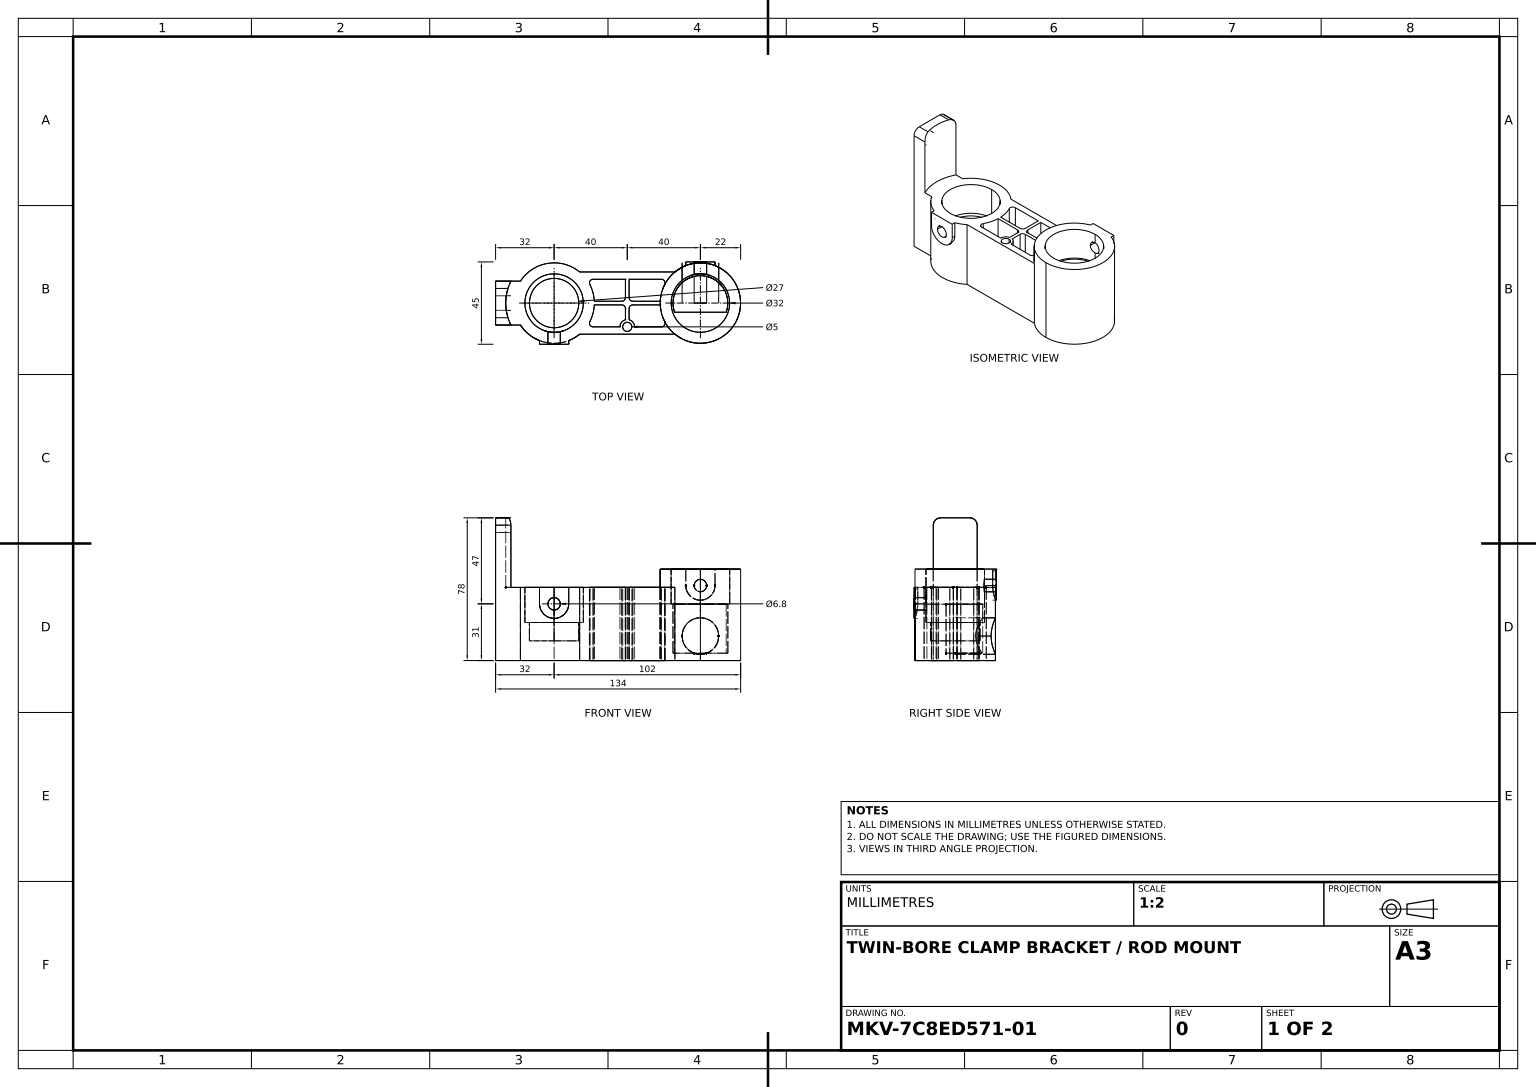
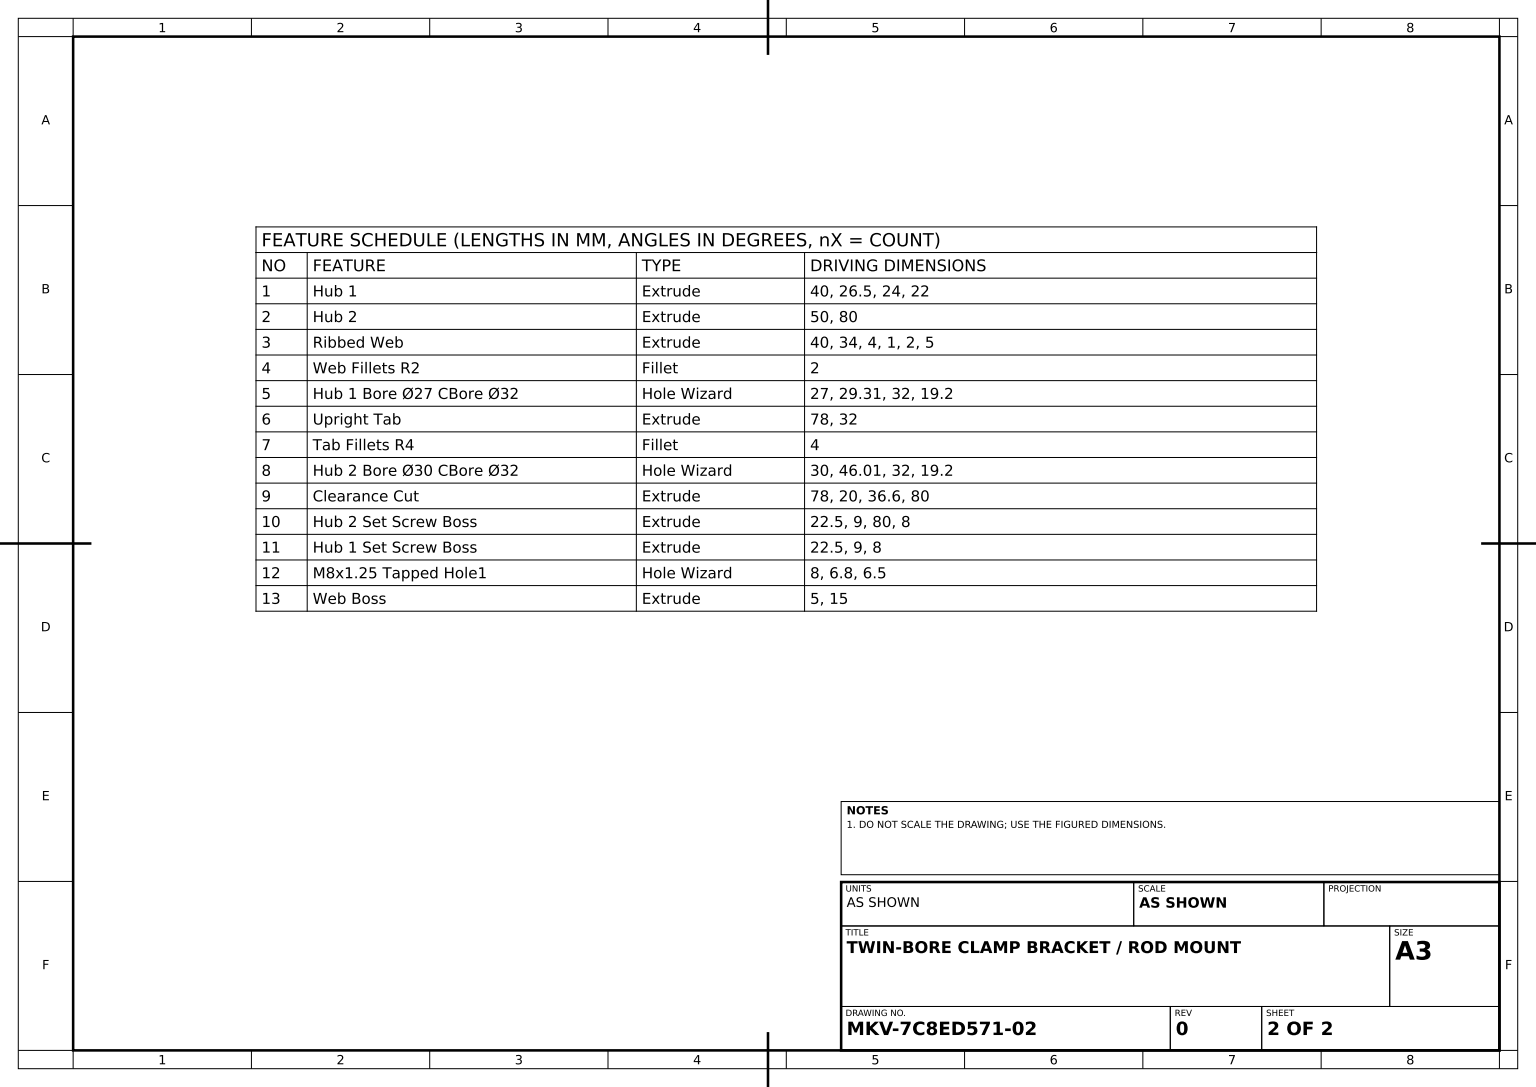
from build123d import *

# Parameters (mm, degrees)
HUB_1_DEPTH                          = 40
HUB_2_SKETCH_R                       = 22
HUB_2_DEPTH                          = 50
RIBBED_WEB_SKETCH_R                  = 2.5
RIBBED_WEB_DEPTH                     = 40
WEB_FILLETS_R2_R                     = 2
HUB_1_BORE_27_CBORE_32_D             = 27
HUB_1_BORE_27_CBORE_32_DEPTH         = 29.20318647
HUB_1_BORE_27_CBORE_32_CBORE_D       = 32
HUB_1_BORE_27_CBORE_32_CBORE_DEPTH   = 19.2
UPRIGHT_TAB_DEPTH                    = 78
TAB_FILLETS_R4_R                     = 4
HUB_2_BORE_30_CBORE_32_D             = 30
HUB_2_BORE_30_CBORE_32_DEPTH         = 45.999131514
HUB_2_BORE_30_CBORE_32_CBORE_D       = 32
HUB_2_BORE_30_CBORE_32_CBORE_DEPTH   = 19.2
CLEARANCE_CUT_SKETCH_R               = 10
CLEARANCE_CUT_DEPTH                  = 78
HUB_2_SET_SCREW_BOSS_REACH           = 137.898
HUB_2_SET_SCREW_BOSS_END_RADIUS      = 22
HUB_1_SET_SCREW_BOSS_REACH           = 138.062
HUB_1_SET_SCREW_BOSS_END_RADIUS      = 22
M8X1_25_TAPPED_HOLE1_REACH           = 129.475
M8X1_25_TAPPED_HOLE1_BORE_R          = 3.4
M8X1_25_TAPPED_HOLE1_ON_FACE_2_REACH = 122.988
M8X1_25_TAPPED_HOLE1_BORE_2_R        = 3.4
WEB_BOSS_DEPTH                       = 26.799131514


with BuildPart() as part:
    # Hub 1 Sketch → Hub 1 (new body)
    with BuildSketch(Plane(origin=(0, 0, 0), x_dir=(1, 0, 0), z_dir=(0, 1, 0))):
        with BuildLine():
            Line((-23.627314701, 12), (-18.439088915, 12))
            ThreePointArc((-18.439088915, 12), (22, 0), (-18.439088915, -12))
            Line((-18.439088915, -12), (-23.627314701, -12))
            ThreePointArc((-23.627314701, -12), (-26.5, 0), (-23.627314701, 12))
        make_face()
    extrude(amount=HUB_1_DEPTH)



with BuildPart() as body_2:
    # Hub 2 Sketch → Hub 2 (new body)
    with BuildSketch(Plane(origin=(0, 0, 0), x_dir=(1, 0, 0), z_dir=(0, 1, 0))):
        with Locations(Location((80, 0, 0), (0, 0, 270))):
            Circle(HUB_2_SKETCH_R)
    extrude(amount=HUB_2_DEPTH)


with BuildPart() as part_1:
    add(part.part)

    add(body_2.part)  # Ribbed Web merges body 2
    # Ribbed Web Sketch → Ribbed Web (add)
    with BuildSketch(Plane(origin=(0, 0, 0), x_dir=(1, 0, 0), z_dir=(0, 1, 0))):
        with BuildLine():
            Line((39, -1), (39, -9.127016654))
            ThreePointArc((39, -9.127016654), (36.83772234, -10.550510257), (36, -13))
            Line((36, -13), (17.748239349, -13))
            ThreePointArc((17.748239349, -13), (15.981875275, -15.118851236), (13.964240044, -17))
            Line((13.964240044, -17), (66.035759956, -17))
            ThreePointArc((66.035759956, -17), (64.018124725, -15.118851236), (62.251760651, -13))
            Line((62.251760651, -13), (44, -13))
            ThreePointArc((44, -13), (43.16227766, -10.550510257), (41, -9.127016654))
            Line((41, -9.127016654), (41, -1))
            Line((41, -1), (58.022739024, -1))
            ThreePointArc((58.022739024, -1), (58, 0), (58.022739024, 1))
            Line((58.022739024, 1), (41, 1))
            Line((41, 1), (41, 13))
            Line((41, 13), (62.251760651, 13))
            ThreePointArc((62.251760651, 13), (64.018124725, 15.118851236), (66.035759956, 17))
            Line((66.035759956, 17), (13.964240044, 17))
            ThreePointArc((13.964240044, 17), (15.981875275, 15.118851236), (17.748239349, 13))
            Line((17.748239349, 13), (39, 13))
            Line((39, 13), (39, 1))
            Line((39, 1), (21.977260976, 1))
            ThreePointArc((21.977260976, 1), (22, 0), (21.977260976, -1))
            Line((21.977260976, -1), (39, -1))
        make_face()
        with Locations(Location((40, -13, 0), (0, 0, 270))):
            Circle(RIBBED_WEB_SKETCH_R, mode=Mode.SUBTRACT)
    extrude(amount=RIBBED_WEB_DEPTH)

    # Web Fillets R2
    web_fillets_r2_edges = [part_1.edges().sort_by_distance(p)[0] for p in [
        (39, 20, 1),
        (17.748239349, 20, 13),
        (62.251760651, 20, 13),
        (41, 20, 1),
        (41, 20, -1),
        (62.251760651, 20, -13),
        (17.748239349, 20, -13),
        (39, 20, -1),
    ]]
    fillet(web_fillets_r2_edges, radius=WEB_FILLETS_R2_R)

    # Hub 1 Bore Ø27 CBore Ø32
    with Locations(Plane.ZX.offset(40)):
        with Locations((0, 0)):
            CounterBoreHole(HUB_1_BORE_27_CBORE_32_D / 2, HUB_1_BORE_27_CBORE_32_CBORE_D / 2, HUB_1_BORE_27_CBORE_32_CBORE_DEPTH, depth=HUB_1_BORE_27_CBORE_32_DEPTH)

    # Upright Tab Sketch → Upright Tab (add)
    with BuildSketch(Plane(origin=(0, 0, 0), x_dir=(1, 0, 0), z_dir=(0, 1, 0))):
        with BuildLine():
            Line((-23.627314701, 12), (-32, 12))
            Line((-32, 12), (-32, -12))
            Line((-32, -12), (-23.627314701, -12))
            ThreePointArc((-23.627314701, -12), (-26.5, 0), (-23.627314701, 12))
        make_face()
    extrude(amount=UPRIGHT_TAB_DEPTH)

    # Tab Fillets R4
    tab_fillets_r4_edges = [part_1.edges().sort_by_distance(p)[0] for p in [
        (-27.813657351, 78, -12),
        (-27.813657351, 78, 12),
    ]]
    fillet(tab_fillets_r4_edges, radius=TAB_FILLETS_R4_R)

    # Hub 2 Bore Ø30 CBore Ø32
    with Locations(Plane(origin=(80, 50, 0), x_dir=(0, 0, 1), z_dir=(0, 1, 0))):
        with Locations((0, 0)):
            CounterBoreHole(HUB_2_BORE_30_CBORE_32_D / 2, HUB_2_BORE_30_CBORE_32_CBORE_D / 2, HUB_2_BORE_30_CBORE_32_CBORE_DEPTH, depth=HUB_2_BORE_30_CBORE_32_DEPTH)

    # Clearance Cut Sketch → Clearance Cut (cut)
    with BuildSketch(Plane.XY):
        with Locations(Location((80, 13.4, 0), (0, 0, 289.963023571))):
            Circle(CLEARANCE_CUT_SKETCH_R)
    extrude(amount=-CLEARANCE_CUT_DEPTH, mode=Mode.SUBTRACT)

    # Hub 2 Set Screw Boss: up to this cylinder (the profile starts outside it)
    hub_2_set_screw_boss_end = Plane(origin=(80, 42.254102, 0), z_dir=(0, -1, 0)) * Cylinder(HUB_2_SET_SCREW_BOSS_END_RADIUS, 320.796, mode=Mode.PRIVATE)
    # Hub 2 Set Screw Boss Sketch → Hub 2 Set Screw Boss (add, up to the surface)
    with BuildSketch(Plane.XY.offset(-22.5), mode=Mode.PRIVATE) as hub_2_set_screw_boss_sk1:
        with BuildLine():
            Line((72, 41), (72, 50))
            Line((72, 50), (88, 50))
            Line((88, 50), (88, 41))
            ThreePointArc((88, 41), (80, 33), (72, 41))
        make_face()
    hub_2_set_screw_boss_tool1 = extrude(hub_2_set_screw_boss_sk1.sketch, amount=HUB_2_SET_SCREW_BOSS_REACH, mode=Mode.PRIVATE) - hub_2_set_screw_boss_end
    add(hub_2_set_screw_boss_tool1.solids().sort_by_distance((80, 42.254102, -22.5))[0])

    # Hub 1 Set Screw Boss: up to this cylinder (the profile starts outside it)
    hub_1_set_screw_boss_end = Plane(origin=(0, 32.254102, 0), z_dir=(0, -1, 0)) * Cylinder(HUB_1_SET_SCREW_BOSS_END_RADIUS, 321.124, mode=Mode.PRIVATE)
    # Hub 1 Set Screw Boss Sketch → Hub 1 Set Screw Boss (add, up to the surface)
    with BuildSketch(Plane.XY.offset(22.5), mode=Mode.PRIVATE) as hub_1_set_screw_boss_sk1:
        with BuildLine():
            Line((-8, 31), (-8, 40))
            Line((-8, 40), (8, 40))
            Line((8, 40), (8, 31))
            ThreePointArc((8, 31), (0, 23), (-8, 31))
        make_face()
    hub_1_set_screw_boss_tool1 = extrude(hub_1_set_screw_boss_sk1.sketch, amount=-HUB_1_SET_SCREW_BOSS_REACH, mode=Mode.PRIVATE) - hub_1_set_screw_boss_end
    add(hub_1_set_screw_boss_tool1.solids().sort_by_distance((0, 32.254102, 22.5))[0])

    # M8x1.25 Tapped Hole1 bore (on position points) → M8x1.25 Tapped Hole1 (cut, up to next)
    with BuildSketch(Plane(origin=(80, 41, -22.5), x_dir=(-1, 0, 0), z_dir=(0, 0, -1)), mode=Mode.PRIVATE) as m8x1_25_tapped_hole1_sk1:
        Circle(M8X1_25_TAPPED_HOLE1_BORE_R)
    m8x1_25_tapped_hole1_tool1 = extrude(m8x1_25_tapped_hole1_sk1.sketch, amount=-M8X1_25_TAPPED_HOLE1_REACH, mode=Mode.PRIVATE) & part_1.part
    add(m8x1_25_tapped_hole1_tool1.solids().sort_by_distance((80, 41, -22.5))[0], mode=Mode.SUBTRACT)

    # M8x1.25 Tapped Hole1 bore 2 (on position points) → M8x1.25 Tapped Hole1 on face 2 (cut, up to next)
    with BuildSketch(Plane(origin=(0, 31, 22.5), x_dir=(1, 0, 0), z_dir=(0, 0, 1)), mode=Mode.PRIVATE) as m8x1_25_tapped_hole1_on_face_2_sk1:
        Circle(M8X1_25_TAPPED_HOLE1_BORE_2_R)
    m8x1_25_tapped_hole1_on_face_2_tool1 = extrude(m8x1_25_tapped_hole1_on_face_2_sk1.sketch, amount=-M8X1_25_TAPPED_HOLE1_ON_FACE_2_REACH, mode=Mode.PRIVATE) & part_1.part
    add(m8x1_25_tapped_hole1_on_face_2_tool1.solids().sort_by_distance((0, 31, 22.5))[0], mode=Mode.SUBTRACT)

    # Web Boss Sketch → Web Boss (add)
    with BuildSketch(Plane(origin=(0, 4.000868486, 0), x_dir=(1, 0, 0), z_dir=(0, 1, 0))):
        with BuildLine():
            Line((65.857864376, -5), (94.142135624, -5))
            ThreePointArc((94.142135624, -5), (80, -15), (65.857864376, -5))
        make_face()
    extrude(amount=WEB_BOSS_DEPTH)


solid = part_1.part
